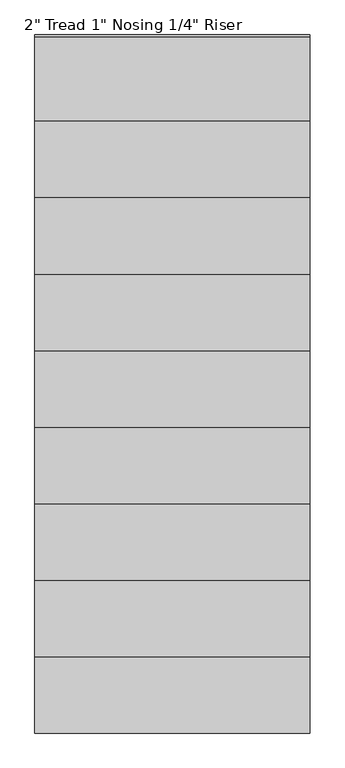
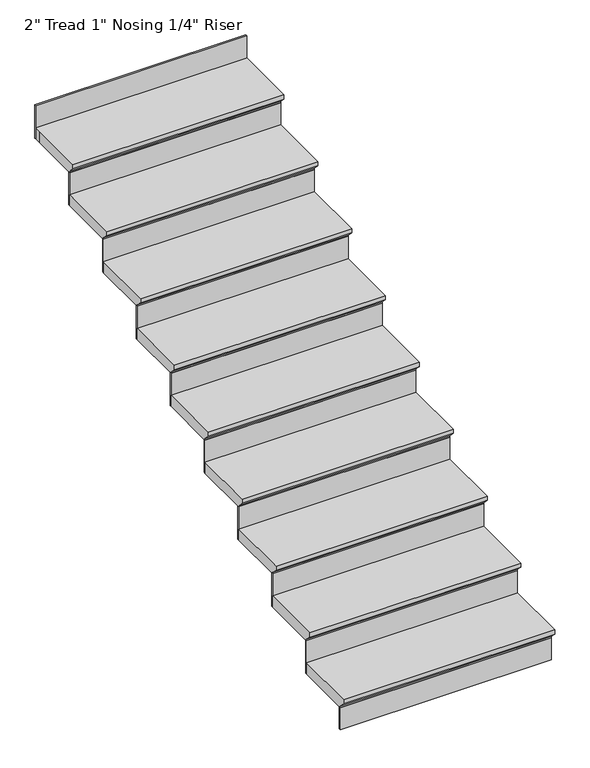
"""IFC4 building model written with IfcOpenShell, lengths in millimetres: stair flight geometry."""

from ifc_helpers import new_model, si_unit, origin, place, context, project, spatial, faceted_brep, source, transform, mapped, element, save


def stair_flight_7beec1f7(model_context):
    return source(origin(), model_context, "Body", "Brep", [
        faceted_brep([(-9627.8771954, -4957.4727897, 133.35), (-9627.8771954, -4957.4727897, 152.4), (-10542.2771954, -4957.4727897, 152.4), (-10542.2771954, -4957.4727897, 133.35), (-9627.8771954, -4932.0727897, 107.95), (-10542.2771954, -4932.0727897, 107.95), (-9627.8771954, -4678.0727897, 152.4), (-10542.2771954, -4678.0727897, 152.4), (-10542.2771954, -4932.0727897, 101.6), (-10542.2771954, -4678.0727897, 101.6), (-9627.8771954, -4678.0727897, 101.6), (-9627.8771954, -4932.0727897, 101.6)], [[[0, 1, 2, 3]], [[4, 0, 3, 5]], [[2, 1, 6, 7]], [[8, 9, 10, 11]], [[2, 7, 9, 8, 5, 3]], [[8, 11, 4, 5]], [[6, 1, 0, 4, 11, 10]], [[7, 6, 10, 9]]]),
        faceted_brep([(-9627.8771954, -4932.0727897, 101.6), (-9627.8771954, -4932.0727897, 0.0), (-9627.8771954, -4925.7227897, 0.0), (-9627.8771954, -4925.7227897, 101.6), (-10542.2771954, -4932.0727897, 101.6), (-10542.2771954, -4925.7227897, 101.6), (-10542.2771954, -4925.7227897, 0.0), (-10542.2771954, -4932.0727897, 0.0)], [[[0, 1, 2, 3]], [[4, 5, 6, 7]], [[1, 0, 4, 7]], [[2, 1, 7, 6]], [[3, 2, 6, 5]], [[0, 3, 5, 4]]]),
        faceted_brep([(-9627.8771954, -4678.0727897, 254.0), (-9627.8771954, -4678.0727897, 101.6), (-9627.8771954, -4671.7227897, 101.6), (-9627.8771954, -4671.7227897, 254.0), (-10542.2771954, -4678.0727897, 254.0), (-10542.2771954, -4671.7227897, 254.0), (-10542.2771954, -4671.7227897, 101.6), (-10542.2771954, -4678.0727897, 101.6)], [[[0, 1, 2, 3]], [[4, 5, 6, 7]], [[1, 0, 4, 7]], [[2, 1, 7, 6]], [[3, 2, 6, 5]], [[0, 3, 5, 4]]]),
        faceted_brep([(-10542.2771954, -4703.4727897, 304.8), (-9627.8771954, -4703.4727897, 304.8), (-9627.8771954, -4424.0727897, 304.8), (-10542.2771954, -4424.0727897, 304.8), (-10542.2771954, -4678.0727897, 254.0), (-10542.2771954, -4424.0727897, 254.0), (-9627.8771954, -4424.0727897, 254.0), (-9627.8771954, -4678.0727897, 254.0), (-10542.2771954, -4678.0727897, 260.35), (-10542.2771954, -4703.4727897, 285.75), (-9627.8771954, -4678.0727897, 260.35), (-9627.8771954, -4703.4727897, 285.75)], [[[0, 1, 2, 3]], [[4, 5, 6, 7]], [[0, 3, 5, 4, 8, 9]], [[4, 7, 10, 8]], [[2, 1, 11, 10, 7, 6]], [[3, 2, 6, 5]], [[11, 1, 0, 9]], [[10, 11, 9, 8]]]),
        faceted_brep([(-9627.8771954, -4424.0727897, 406.4), (-9627.8771954, -4424.0727897, 254.0), (-9627.8771954, -4417.7227897, 254.0), (-9627.8771954, -4417.7227897, 406.4), (-10542.2771954, -4424.0727897, 406.4), (-10542.2771954, -4417.7227897, 406.4), (-10542.2771954, -4417.7227897, 254.0), (-10542.2771954, -4424.0727897, 254.0)], [[[0, 1, 2, 3]], [[4, 5, 6, 7]], [[1, 0, 4, 7]], [[2, 1, 7, 6]], [[3, 2, 6, 5]], [[0, 3, 5, 4]]]),
        faceted_brep([(-10542.2771954, -4449.4727897, 457.2), (-9627.8771954, -4449.4727897, 457.2), (-9627.8771954, -4170.0727897, 457.2), (-10542.2771954, -4170.0727897, 457.2), (-10542.2771954, -4424.0727897, 406.4), (-10542.2771954, -4170.0727897, 406.4), (-9627.8771954, -4170.0727897, 406.4), (-9627.8771954, -4424.0727897, 406.4), (-10542.2771954, -4424.0727897, 412.75), (-10542.2771954, -4449.4727897, 438.15), (-9627.8771954, -4424.0727897, 412.75), (-9627.8771954, -4449.4727897, 438.15)], [[[0, 1, 2, 3]], [[4, 5, 6, 7]], [[0, 3, 5, 4, 8, 9]], [[4, 7, 10, 8]], [[2, 1, 11, 10, 7, 6]], [[3, 2, 6, 5]], [[11, 1, 0, 9]], [[10, 11, 9, 8]]]),
        faceted_brep([(-9627.8771954, -4170.0727897, 558.8), (-9627.8771954, -4170.0727897, 406.4), (-9627.8771954, -4163.7227897, 406.4), (-9627.8771954, -4163.7227897, 558.8), (-10542.2771954, -4170.0727897, 558.8), (-10542.2771954, -4163.7227897, 558.8), (-10542.2771954, -4163.7227897, 406.4), (-10542.2771954, -4170.0727897, 406.4)], [[[0, 1, 2, 3]], [[4, 5, 6, 7]], [[1, 0, 4, 7]], [[2, 1, 7, 6]], [[3, 2, 6, 5]], [[0, 3, 5, 4]]]),
        faceted_brep([(-10542.2771954, -4195.4727897, 609.6), (-9627.8771954, -4195.4727897, 609.6), (-9627.8771954, -3916.0727897, 609.6), (-10542.2771954, -3916.0727897, 609.6), (-10542.2771954, -4170.0727897, 558.8), (-10542.2771954, -3916.0727897, 558.8), (-9627.8771954, -3916.0727897, 558.8), (-9627.8771954, -4170.0727897, 558.8), (-10542.2771954, -4170.0727897, 565.15), (-10542.2771954, -4195.4727897, 590.55), (-9627.8771954, -4170.0727897, 565.15), (-9627.8771954, -4195.4727897, 590.55)], [[[0, 1, 2, 3]], [[4, 5, 6, 7]], [[0, 3, 5, 4, 8, 9]], [[4, 7, 10, 8]], [[2, 1, 11, 10, 7, 6]], [[3, 2, 6, 5]], [[11, 1, 0, 9]], [[10, 11, 9, 8]]]),
        faceted_brep([(-9627.8771954, -3916.0727897, 711.2), (-9627.8771954, -3916.0727897, 558.8), (-9627.8771954, -3909.7227897, 558.8), (-9627.8771954, -3909.7227897, 711.2), (-10542.2771954, -3916.0727897, 711.2), (-10542.2771954, -3909.7227897, 711.2), (-10542.2771954, -3909.7227897, 558.8), (-10542.2771954, -3916.0727897, 558.8)], [[[0, 1, 2, 3]], [[4, 5, 6, 7]], [[1, 0, 4, 7]], [[2, 1, 7, 6]], [[3, 2, 6, 5]], [[0, 3, 5, 4]]]),
        faceted_brep([(-10542.2771954, -3941.4727897, 762.0), (-9627.8771954, -3941.4727897, 762.0), (-9627.8771954, -3662.0727897, 762.0), (-10542.2771954, -3662.0727897, 762.0), (-10542.2771954, -3916.0727897, 711.2), (-10542.2771954, -3662.0727897, 711.2), (-9627.8771954, -3662.0727897, 711.2), (-9627.8771954, -3916.0727897, 711.2), (-10542.2771954, -3916.0727897, 717.55), (-10542.2771954, -3941.4727897, 742.95), (-9627.8771954, -3916.0727897, 717.55), (-9627.8771954, -3941.4727897, 742.95)], [[[0, 1, 2, 3]], [[4, 5, 6, 7]], [[0, 3, 5, 4, 8, 9]], [[4, 7, 10, 8]], [[2, 1, 11, 10, 7, 6]], [[3, 2, 6, 5]], [[11, 1, 0, 9]], [[10, 11, 9, 8]]]),
        faceted_brep([(-9627.8771954, -3662.0727897, 863.6), (-9627.8771954, -3662.0727897, 711.2), (-9627.8771954, -3655.7227897, 711.2), (-9627.8771954, -3655.7227897, 863.6), (-10542.2771954, -3662.0727897, 863.6), (-10542.2771954, -3655.7227897, 863.6), (-10542.2771954, -3655.7227897, 711.2), (-10542.2771954, -3662.0727897, 711.2)], [[[0, 1, 2, 3]], [[4, 5, 6, 7]], [[1, 0, 4, 7]], [[2, 1, 7, 6]], [[3, 2, 6, 5]], [[0, 3, 5, 4]]]),
        faceted_brep([(-10542.2771954, -3687.4727897, 914.4), (-9627.8771954, -3687.4727897, 914.4), (-9627.8771954, -3408.0727897, 914.4), (-10542.2771954, -3408.0727897, 914.4), (-10542.2771954, -3662.0727897, 863.6), (-10542.2771954, -3408.0727897, 863.6), (-9627.8771954, -3408.0727897, 863.6), (-9627.8771954, -3662.0727897, 863.6), (-10542.2771954, -3662.0727897, 869.95), (-10542.2771954, -3687.4727897, 895.35), (-9627.8771954, -3662.0727897, 869.95), (-9627.8771954, -3687.4727897, 895.35)], [[[0, 1, 2, 3]], [[4, 5, 6, 7]], [[0, 3, 5, 4, 8, 9]], [[4, 7, 10, 8]], [[2, 1, 11, 10, 7, 6]], [[3, 2, 6, 5]], [[11, 1, 0, 9]], [[10, 11, 9, 8]]]),
        faceted_brep([(-9627.8771954, -3408.0727897, 1016.0), (-9627.8771954, -3408.0727897, 863.6), (-9627.8771954, -3401.7227897, 863.6), (-9627.8771954, -3401.7227897, 1016.0), (-10542.2771954, -3408.0727897, 1016.0), (-10542.2771954, -3401.7227897, 1016.0), (-10542.2771954, -3401.7227897, 863.6), (-10542.2771954, -3408.0727897, 863.6)], [[[0, 1, 2, 3]], [[4, 5, 6, 7]], [[1, 0, 4, 7]], [[2, 1, 7, 6]], [[3, 2, 6, 5]], [[0, 3, 5, 4]]]),
        faceted_brep([(-10542.2771954, -3433.4727897, 1066.8), (-9627.8771954, -3433.4727897, 1066.8), (-9627.8771954, -3154.0727897, 1066.8), (-10542.2771954, -3154.0727897, 1066.8), (-10542.2771954, -3408.0727897, 1016.0), (-10542.2771954, -3154.0727897, 1016.0), (-9627.8771954, -3154.0727897, 1016.0), (-9627.8771954, -3408.0727897, 1016.0), (-10542.2771954, -3408.0727897, 1022.35), (-10542.2771954, -3433.4727897, 1047.75), (-9627.8771954, -3408.0727897, 1022.35), (-9627.8771954, -3433.4727897, 1047.75)], [[[0, 1, 2, 3]], [[4, 5, 6, 7]], [[0, 3, 5, 4, 8, 9]], [[4, 7, 10, 8]], [[2, 1, 11, 10, 7, 6]], [[3, 2, 6, 5]], [[11, 1, 0, 9]], [[10, 11, 9, 8]]]),
        faceted_brep([(-9627.8771954, -3154.0727897, 1168.4), (-9627.8771954, -3154.0727897, 1016.0), (-9627.8771954, -3147.7227897, 1016.0), (-9627.8771954, -3147.7227897, 1168.4), (-10542.2771954, -3154.0727897, 1168.4), (-10542.2771954, -3147.7227897, 1168.4), (-10542.2771954, -3147.7227897, 1016.0), (-10542.2771954, -3154.0727897, 1016.0)], [[[0, 1, 2, 3]], [[4, 5, 6, 7]], [[1, 0, 4, 7]], [[2, 1, 7, 6]], [[3, 2, 6, 5]], [[0, 3, 5, 4]]]),
        faceted_brep([(-10542.2771954, -3179.4727897, 1219.2), (-9627.8771954, -3179.4727897, 1219.2), (-9627.8771954, -2900.0727897, 1219.2), (-10542.2771954, -2900.0727897, 1219.2), (-10542.2771954, -3154.0727897, 1168.4), (-10542.2771954, -2900.0727897, 1168.4), (-9627.8771954, -2900.0727897, 1168.4), (-9627.8771954, -3154.0727897, 1168.4), (-10542.2771954, -3154.0727897, 1174.75), (-10542.2771954, -3179.4727897, 1200.15), (-9627.8771954, -3154.0727897, 1174.75), (-9627.8771954, -3179.4727897, 1200.15)], [[[0, 1, 2, 3]], [[4, 5, 6, 7]], [[0, 3, 5, 4, 8, 9]], [[4, 7, 10, 8]], [[2, 1, 11, 10, 7, 6]], [[3, 2, 6, 5]], [[11, 1, 0, 9]], [[10, 11, 9, 8]]]),
        faceted_brep([(-9627.8771954, -2646.0727897, 1473.2), (-9627.8771954, -2646.0727897, 1320.8), (-9627.8771954, -2639.7227897, 1320.8), (-9627.8771954, -2639.7227897, 1473.2), (-10542.2771954, -2646.0727897, 1473.2), (-10542.2771954, -2639.7227897, 1473.2), (-10542.2771954, -2639.7227897, 1320.8), (-10542.2771954, -2646.0727897, 1320.8)], [[[0, 1, 2, 3]], [[4, 5, 6, 7]], [[1, 0, 4, 7]], [[2, 1, 7, 6]], [[3, 2, 6, 5]], [[0, 3, 5, 4]]]),
        faceted_brep([(-9627.8771954, -2900.0727897, 1320.8), (-9627.8771954, -2900.0727897, 1168.4), (-9627.8771954, -2893.7227897, 1168.4), (-9627.8771954, -2893.7227897, 1320.8), (-10542.2771954, -2900.0727897, 1320.8), (-10542.2771954, -2893.7227897, 1320.8), (-10542.2771954, -2893.7227897, 1168.4), (-10542.2771954, -2900.0727897, 1168.4)], [[[0, 1, 2, 3]], [[4, 5, 6, 7]], [[1, 0, 4, 7]], [[2, 1, 7, 6]], [[3, 2, 6, 5]], [[0, 3, 5, 4]]]),
        faceted_brep([(-10542.2771954, -2646.0727897, 1371.6), (-10542.2771954, -2671.4727897, 1371.6), (-10542.2771954, -2925.4727897, 1371.6), (-9627.8771954, -2925.4727897, 1371.6), (-9627.8771954, -2671.4727897, 1371.6), (-9627.8771954, -2646.0727897, 1371.6), (-10542.2771954, -2671.4727897, 1320.8), (-10542.2771954, -2646.0727897, 1320.8), (-9627.8771954, -2646.0727897, 1320.8), (-9627.8771954, -2671.4727897, 1320.8), (-9627.8771954, -2900.0727897, 1320.8), (-10542.2771954, -2900.0727897, 1320.8), (-10542.2771954, -2900.0727897, 1327.15), (-10542.2771954, -2925.4727897, 1352.55), (-9627.8771954, -2900.0727897, 1327.15), (-9627.8771954, -2925.4727897, 1352.55)], [[[0, 1, 2, 3, 4, 5]], [[6, 7, 8, 9, 10, 11]], [[1, 0, 7, 6]], [[2, 1, 6, 11, 12, 13]], [[11, 10, 14, 12]], [[4, 3, 15, 14, 10, 9]], [[5, 4, 9, 8]], [[0, 5, 8, 7]], [[15, 3, 2, 13]], [[14, 15, 13, 12]]]),
    ])


if __name__ == "__main__":
    model = new_model("IFC4")
    model_context = context("Model", 3, world=origin())
    ifc_project = project(units=[si_unit("LENGTHUNIT", "METRE", prefix="MILLI")], contexts=[model_context])
    site = spatial("IfcSite", under=ifc_project)
    building = spatial("IfcBuilding", under=site)
    placement = place(None, origin())
    stair_flight_shape = stair_flight_7beec1f7(model_context)
    element("IfcStairFlight", 1, ObjectType="2\" Tread 1\" Nosing 1/4\" Riser", at=placement, inside=building, context=model_context, shape_type="MappedRepresentation", body=[
        mapped(stair_flight_shape, transform((0.0, 0.0, 0.0), x_axis=(1.0, 0.0, 0.0), y_axis=(0.0, 1.0, 0.0), z_axis=(0.0, 0.0, 1.0))),
    ])
    save(model, "model.ifc")
